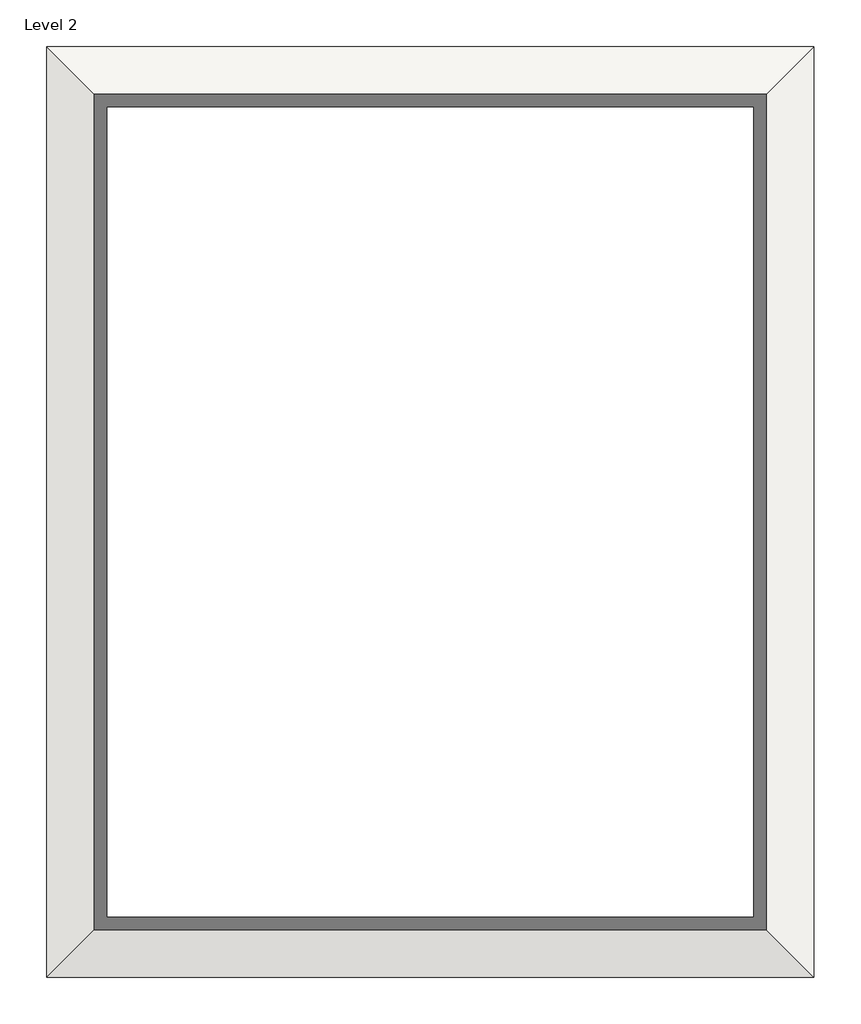
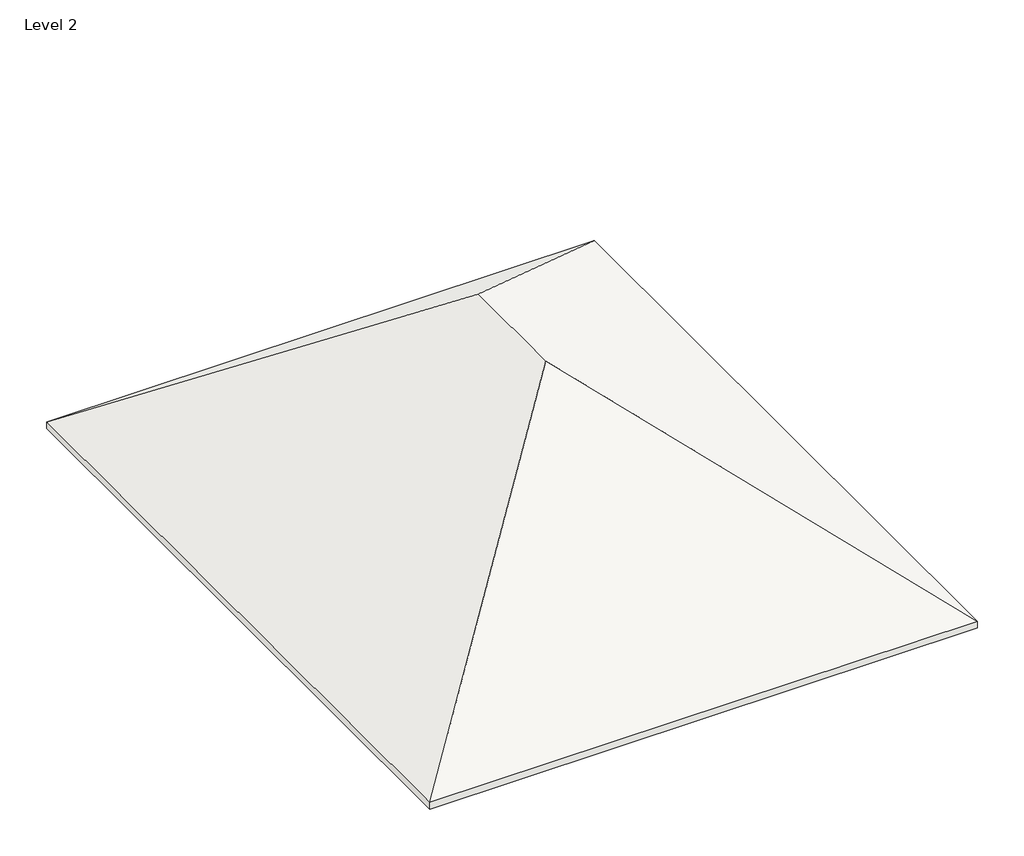
# One storey: 1 roof.
"""IFC4 building model written with IfcOpenShell, lengths in millimetres."""

from ifc_helpers import new_model, si_unit, origin, place, context, project, spatial, faceted_brep, element, save

model = new_model("IFC4")

# Units and contexts
model_context = context("Model", 3, world=origin())
ifc_project = project(units=[si_unit("LENGTHUNIT", "METRE", prefix="MILLI")], contexts=[model_context])

# Site, building, storey
site = spatial("IfcSite", under=ifc_project)
building = spatial("IfcBuilding", under=site)
storey = spatial("IfcBuildingStorey", under=building, Name="Level 2", Elevation=3048.0)

# Roof
placement = place(None, origin())
element("IfcRoof", 1, ObjectType="Wood Rafter 8\" - Asphalt Shingle - Insulated", at=placement, inside=storey, context=model_context, shape_type="Brep", body=[
    faceted_brep([(5603.5704288, 10900.5045891, 3048.0), (-4531.0295712, 765.9045891, 10648.95), (-14665.6295712, 10900.5045891, 3048.0), (5603.5704288, -13686.6954109, 3048.0), (-4531.0295712, -3552.0954109, 10648.95), (-14665.6295712, -13686.6954109, 3048.0), (5603.5704288, 10900.5045891, 3313.90625), (-14665.6295712, 10900.5045891, 3313.90625), (-4531.0295712, 765.9045891, 10914.85625), (-4531.0295712, -3552.0954109, 10914.85625), (5603.5704288, -13686.6954109, 3313.90625), (-14665.6295712, -13686.6954109, 3313.90625)], [[[0, 1, 2]], [[1, 0, 3, 4]], [[5, 4, 3]], [[2, 1, 4, 5]], [[6, 7, 8]], [[6, 8, 9, 10]], [[11, 10, 9]], [[7, 11, 9, 8]], [[2, 7, 6, 0]], [[5, 11, 7, 2]], [[3, 10, 11, 5]], [[0, 6, 10, 3]]]),
])

save(model, "model.ifc")

# Revit data of these elements
# Type "Wood Rafter 8\" - Asphalt Shingle - Insulated"
#   Assembly Code = "B1020"
#   Layers, outside or top first: 0' - 0 1/4" "Asphalt Shingle" (function 4); 0' - 0 5/8" "Plywood, Sheathing" (function 2); 0' - 7 1/2" "Structure, Wood Joist/Rafter Layer, Batt Insulation" (function 1)
# Element 1 (IfcRoof, "Wood Rafter 8\" - Asphalt Shingle - Insulated")
#   built-in parameter 1001705 = 35.8099 (stored number, unit not read)
#   built-in parameter 1001710 = 33615
#   Phase Created = New Construction
#   Materials on its faces: "Structure, Wood Joist/Rafter Layer, Batt Insulation", "Asphalt Shingle"
# Materials
#   "Asphalt Shingle": class "Generic", colour RGB 155 155 155, transparency 0, Description = "Asphalt roofing shingle", Cost = 0
#   "Plywood, Sheathing": class "Wood", colour RGB 212 179 113, transparency 0, Description = "Plywood, sheathing grade", Cost = 0
#   "Structure, Wood Joist/Rafter Layer, Batt Insulation": class "Wood", colour RGB 127 127 127, transparency 0, Description = "Wood framing, insulated", Cost = 0
